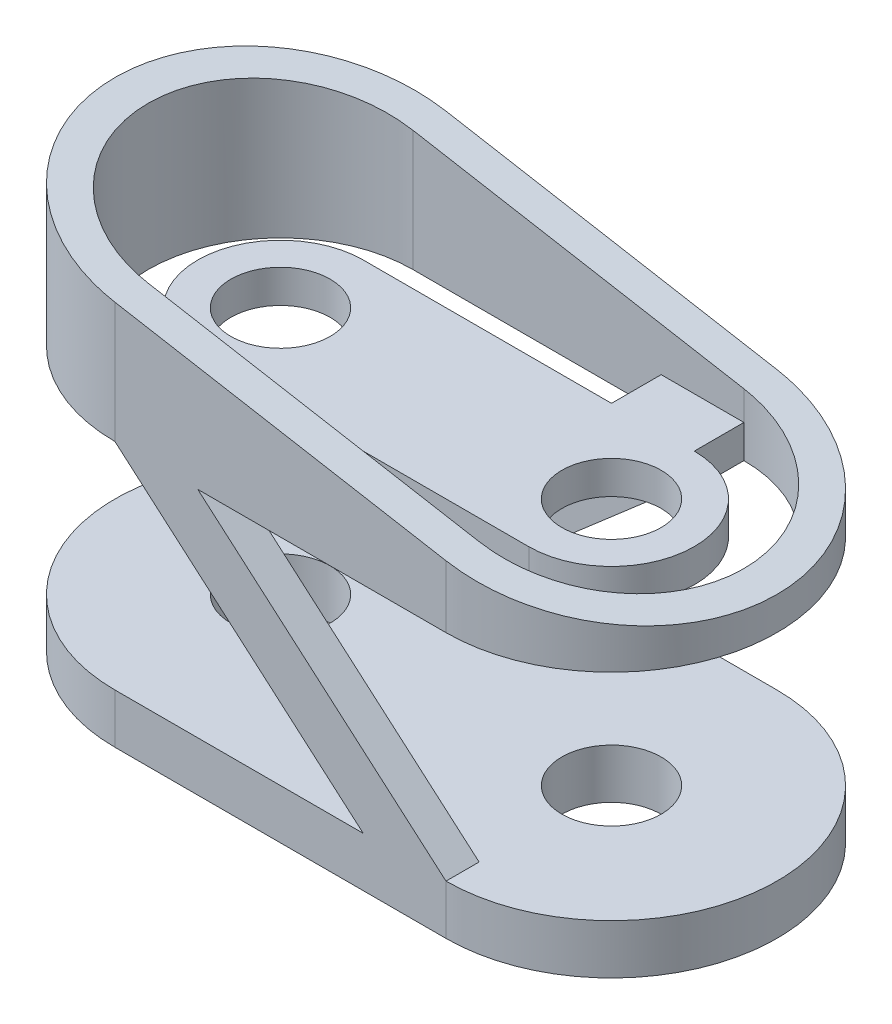
ISO-10303-21;
HEADER;
FILE_DESCRIPTION(('STEP AP214'),'2;1');
FILE_NAME('part.step','',(''),(''),'','','');
FILE_SCHEMA(('AUTOMOTIVE_DESIGN { 1 0 10303 214 1 1 1 1 }'));
ENDSEC;
DATA;
#1=APPLICATION_CONTEXT('core data for automotive mechanical design processes');
#2=APPLICATION_PROTOCOL_DEFINITION('international standard','automotive_design',2000,#1);
#3=PRODUCT_CONTEXT('',#1,'mechanical');
#4=PRODUCT('Part','Part','',(#3));
#5=PRODUCT_RELATED_PRODUCT_CATEGORY('part','',(#4));
#6=PRODUCT_DEFINITION_FORMATION('','',#4);
#7=PRODUCT_DEFINITION_CONTEXT('part definition',#1,'design');
#8=PRODUCT_DEFINITION('design','',#6,#7);
#9=PRODUCT_DEFINITION_SHAPE('','',#8);
#10=(LENGTH_UNIT() NAMED_UNIT(*) SI_UNIT(.MILLI.,.METRE.));
#11=(NAMED_UNIT(*) PLANE_ANGLE_UNIT() SI_UNIT($,.RADIAN.));
#12=(NAMED_UNIT(*) SI_UNIT($,.STERADIAN.) SOLID_ANGLE_UNIT());
#13=UNCERTAINTY_MEASURE_WITH_UNIT(LENGTH_MEASURE(1.E-05),#10,'distance_accuracy_value','');
#14=(GEOMETRIC_REPRESENTATION_CONTEXT(3) GLOBAL_UNCERTAINTY_ASSIGNED_CONTEXT((#13)) GLOBAL_UNIT_ASSIGNED_CONTEXT((#10,
#11,#12)) REPRESENTATION_CONTEXT('',''));
#15=CARTESIAN_POINT('',(0.,0.,0.));
#16=DIRECTION('',(0.,0.,1.));
#17=DIRECTION('',(1.,0.,0.));
#18=AXIS2_PLACEMENT_3D('',#15,#16,#17);
#19=CARTESIAN_POINT('',(-50.,90.,0.));
#20=DIRECTION('',(0.,1.,0.));
#21=DIRECTION('',(0.,0.,1.));
#22=AXIS2_PLACEMENT_3D('',#19,#20,#21);
#23=PLANE('',#22);
#24=CARTESIAN_POINT('',(50.,90.,0.));
#25=DIRECTION('',(0.,-1.,0.));
#26=DIRECTION('',(0.,0.,-1.));
#27=AXIS2_PLACEMENT_3D('',#24,#25,#26);
#28=CIRCLE('',#27,15.);
#29=CARTESIAN_POINT('',(50.,90.,-15.));
#30=VERTEX_POINT('',#29);
#31=EDGE_CURVE('E246',#30,#30,#28,.T.);
#32=ORIENTED_EDGE('',*,*,#31,.T.);
#33=EDGE_LOOP('',(#32));
#34=FACE_BOUND('',#33,.T.);
#35=CARTESIAN_POINT('',(-50.,90.,0.));
#36=DIRECTION('',(0.,-1.,0.));
#37=DIRECTION('',(0.,0.,-1.));
#38=AXIS2_PLACEMENT_3D('',#35,#36,#37);
#39=CIRCLE('',#38,15.);
#40=CARTESIAN_POINT('',(-50.,90.,-15.));
#41=VERTEX_POINT('',#40);
#42=EDGE_CURVE('E238',#41,#41,#39,.T.);
#43=ORIENTED_EDGE('',*,*,#42,.T.);
#44=EDGE_LOOP('',(#43));
#45=FACE_BOUND('',#44,.T.);
#46=DIRECTION('',(0.,0.,1.));
#47=VECTOR('',#46,1.);
#48=CARTESIAN_POINT('',(50.,90.,-25.));
#49=LINE('',#48,#47);
#50=CARTESIAN_POINT('',(50.,90.,-40.));
#51=VERTEX_POINT('',#50);
#52=CARTESIAN_POINT('',(50.,90.,-25.));
#53=VERTEX_POINT('',#52);
#54=EDGE_CURVE('E273',#51,#53,#49,.T.);
#55=ORIENTED_EDGE('',*,*,#54,.F.);
#56=DIRECTION('',(-1.,0.,0.));
#57=VECTOR('',#56,1.);
#58=CARTESIAN_POINT('',(50.,90.,-40.));
#59=LINE('',#58,#57);
#60=CARTESIAN_POINT('',(25.,90.,-40.));
#61=VERTEX_POINT('',#60);
#62=EDGE_CURVE('E237',#51,#61,#59,.T.);
#63=ORIENTED_EDGE('',*,*,#62,.T.);
#64=DIRECTION('',(0.,0.,-1.));
#65=VECTOR('',#64,1.);
#66=CARTESIAN_POINT('',(25.,90.,-25.));
#67=LINE('',#66,#65);
#68=CARTESIAN_POINT('',(25.,90.,-25.));
#69=VERTEX_POINT('',#68);
#70=EDGE_CURVE('E271',#69,#61,#67,.T.);
#71=ORIENTED_EDGE('',*,*,#70,.F.);
#72=DIRECTION('',(1.,0.,0.));
#73=VECTOR('',#72,1.);
#74=CARTESIAN_POINT('',(25.,90.,-25.));
#75=LINE('',#74,#73);
#76=CARTESIAN_POINT('',(-50.,90.,-25.));
#77=VERTEX_POINT('',#76);
#78=EDGE_CURVE('E268',#77,#69,#75,.T.);
#79=ORIENTED_EDGE('',*,*,#78,.F.);
#80=CARTESIAN_POINT('',(-50.,90.,0.));
#81=DIRECTION('',(0.,-1.,0.));
#82=DIRECTION('',(0.,0.,-1.));
#83=AXIS2_PLACEMENT_3D('',#80,#81,#82);
#84=CIRCLE('',#83,25.);
#85=CARTESIAN_POINT('',(-50.,90.,25.));
#86=VERTEX_POINT('',#85);
#87=EDGE_CURVE('E264',#86,#77,#84,.T.);
#88=ORIENTED_EDGE('',*,*,#87,.F.);
#89=DIRECTION('',(0.,0.,-1.));
#90=VECTOR('',#89,1.);
#91=CARTESIAN_POINT('',(-50.,90.,25.));
#92=LINE('',#91,#90);
#93=CARTESIAN_POINT('',(-50.,90.,40.));
#94=VERTEX_POINT('',#93);
#95=EDGE_CURVE('E265',#94,#86,#92,.T.);
#96=ORIENTED_EDGE('',*,*,#95,.F.);
#97=DIRECTION('',(1.,0.,0.));
#98=VECTOR('',#97,1.);
#99=CARTESIAN_POINT('',(50.,90.,40.));
#100=LINE('',#99,#98);
#101=CARTESIAN_POINT('',(-25.,90.,40.));
#102=VERTEX_POINT('',#101);
#103=EDGE_CURVE('E235',#94,#102,#100,.T.);
#104=ORIENTED_EDGE('',*,*,#103,.T.);
#105=DIRECTION('',(0.,0.,1.));
#106=VECTOR('',#105,1.);
#107=CARTESIAN_POINT('',(-25.,90.,40.));
#108=LINE('',#107,#106);
#109=CARTESIAN_POINT('',(-25.,90.,25.));
#110=VERTEX_POINT('',#109);
#111=EDGE_CURVE('E259',#110,#102,#108,.T.);
#112=ORIENTED_EDGE('',*,*,#111,.F.);
#113=DIRECTION('',(-1.,0.,0.));
#114=VECTOR('',#113,1.);
#115=CARTESIAN_POINT('',(50.,90.,25.));
#116=LINE('',#115,#114);
#117=CARTESIAN_POINT('',(50.,90.,25.));
#118=VERTEX_POINT('',#117);
#119=EDGE_CURVE('E254',#118,#110,#116,.T.);
#120=ORIENTED_EDGE('',*,*,#119,.F.);
#121=CARTESIAN_POINT('',(50.,90.,0.));
#122=DIRECTION('',(0.,-1.,0.));
#123=DIRECTION('',(0.,0.,-1.));
#124=AXIS2_PLACEMENT_3D('',#121,#122,#123);
#125=CIRCLE('',#124,25.);
#126=EDGE_CURVE('E252',#53,#118,#125,.T.);
#127=ORIENTED_EDGE('',*,*,#126,.F.);
#128=EDGE_LOOP('',(#55,#63,#71,#79,#88,#96,#104,#112,#120,#127));
#129=FACE_BOUND('',#128,.T.);
#130=ADVANCED_FACE('F39',(#34,#45,#129),#23,.T.);
#131=CARTESIAN_POINT('',(-50.,90.,40.));
#132=DIRECTION('',(0.,0.,-1.));
#133=DIRECTION('',(-1.,0.,0.));
#134=AXIS2_PLACEMENT_3D('',#131,#132,#133);
#135=PLANE('',#134);
#136=DIRECTION('',(0.,-1.,0.));
#137=VECTOR('',#136,1.);
#138=CARTESIAN_POINT('',(-25.,90.,40.));
#139=LINE('',#138,#137);
#140=CARTESIAN_POINT('',(-25.,80.,40.));
#141=VERTEX_POINT('',#140);
#142=EDGE_CURVE('E320',#102,#141,#139,.T.);
#143=ORIENTED_EDGE('',*,*,#142,.F.);
#144=ORIENTED_EDGE('',*,*,#103,.F.);
#145=DIRECTION('',(0.,-1.,0.));
#146=VECTOR('',#145,1.);
#147=CARTESIAN_POINT('',(-50.,332.964243462777,40.));
#148=LINE('',#147,#146);
#149=CARTESIAN_POINT('',(-50.,116.44904710627,40.));
#150=VERTEX_POINT('',#149);
#151=EDGE_CURVE('E221',#150,#94,#148,.T.);
#152=ORIENTED_EDGE('',*,*,#151,.F.);
#153=DIRECTION('',(0.984807753012208,-0.173648177666931,0.));
#154=VECTOR('',#153,1.);
#155=CARTESIAN_POINT('',(9.95835179427637,105.876771966129,40.));
#156=LINE('',#155,#154);
#157=CARTESIAN_POINT('',(50.,98.8163490354233,40.));
#158=VERTEX_POINT('',#157);
#159=EDGE_CURVE('E206',#150,#158,#156,.T.);
#160=ORIENTED_EDGE('',*,*,#159,.T.);
#161=DIRECTION('',(0.,-1.,0.));
#162=VECTOR('',#161,1.);
#163=CARTESIAN_POINT('',(50.,90.,40.));
#164=LINE('',#163,#162);
#165=CARTESIAN_POINT('',(50.,80.,40.));
#166=VERTEX_POINT('',#165);
#167=EDGE_CURVE('E356',#158,#166,#164,.T.);
#168=ORIENTED_EDGE('',*,*,#167,.T.);
#169=DIRECTION('',(1.,0.,0.));
#170=VECTOR('',#169,1.);
#171=CARTESIAN_POINT('',(-50.,80.,40.));
#172=LINE('',#171,#170);
#173=EDGE_CURVE('E344',#141,#166,#172,.T.);
#174=ORIENTED_EDGE('',*,*,#173,.F.);
#175=EDGE_LOOP('',(#143,#144,#152,#160,#168,#174));
#176=FACE_BOUND('',#175,.T.);
#177=ADVANCED_FACE('F231',(#176),#135,.T.);
#178=CARTESIAN_POINT('',(-50.,90.,-40.));
#179=DIRECTION('',(0.,0.,1.));
#180=DIRECTION('',(1.,0.,0.));
#181=AXIS2_PLACEMENT_3D('',#178,#179,#180);
#182=PLANE('',#181);
#183=DIRECTION('',(0.,-1.,0.));
#184=VECTOR('',#183,1.);
#185=CARTESIAN_POINT('',(25.,90.,-40.));
#186=LINE('',#185,#184);
#187=CARTESIAN_POINT('',(25.,80.,-40.));
#188=VERTEX_POINT('',#187);
#189=EDGE_CURVE('E306',#61,#188,#186,.T.);
#190=ORIENTED_EDGE('',*,*,#189,.F.);
#191=ORIENTED_EDGE('',*,*,#62,.F.);
#192=DIRECTION('',(0.,-1.,0.));
#193=VECTOR('',#192,1.);
#194=CARTESIAN_POINT('',(50.,332.964243462777,-40.));
#195=LINE('',#194,#193);
#196=CARTESIAN_POINT('',(50.,98.8163490354233,-40.));
#197=VERTEX_POINT('',#196);
#198=EDGE_CURVE('E217',#197,#51,#195,.T.);
#199=ORIENTED_EDGE('',*,*,#198,.F.);
#200=DIRECTION('',(-0.984807753012208,0.173648177666931,0.));
#201=VECTOR('',#200,1.);
#202=CARTESIAN_POINT('',(9.95835179427632,105.876771966129,-40.));
#203=LINE('',#202,#201);
#204=CARTESIAN_POINT('',(-50.,116.44904710627,-40.));
#205=VERTEX_POINT('',#204);
#206=EDGE_CURVE('E226',#197,#205,#203,.T.);
#207=ORIENTED_EDGE('',*,*,#206,.T.);
#208=DIRECTION('',(0.,-1.,0.));
#209=VECTOR('',#208,1.);
#210=CARTESIAN_POINT('',(-50.,90.,-40.));
#211=LINE('',#210,#209);
#212=CARTESIAN_POINT('',(-50.,80.,-40.));
#213=VERTEX_POINT('',#212);
#214=EDGE_CURVE('E230',#205,#213,#211,.T.);
#215=ORIENTED_EDGE('',*,*,#214,.T.);
#216=DIRECTION('',(-1.,0.,0.));
#217=VECTOR('',#216,1.);
#218=CARTESIAN_POINT('',(-50.,80.,-40.));
#219=LINE('',#218,#217);
#220=EDGE_CURVE('E348',#188,#213,#219,.T.);
#221=ORIENTED_EDGE('',*,*,#220,.F.);
#222=EDGE_LOOP('',(#190,#191,#199,#207,#215,#221));
#223=FACE_BOUND('',#222,.T.);
#224=ADVANCED_FACE('F502',(#223),#182,.T.);
#225=CARTESIAN_POINT('',(-50.,80.,0.));
#226=DIRECTION('',(0.,1.,0.));
#227=DIRECTION('',(0.,0.,1.));
#228=AXIS2_PLACEMENT_3D('',#225,#226,#227);
#229=PLANE('',#228);
#230=CARTESIAN_POINT('',(50.,80.,0.));
#231=DIRECTION('',(0.,1.,0.));
#232=DIRECTION('',(0.,0.,1.));
#233=AXIS2_PLACEMENT_3D('',#230,#231,#232);
#234=CIRCLE('',#233,40.);
#235=CARTESIAN_POINT('',(50.0000000000004,80.,-40.));
#236=VERTEX_POINT('',#235);
#237=EDGE_CURVE('E350',#166,#236,#234,.T.);
#238=ORIENTED_EDGE('',*,*,#237,.T.);
#239=DIRECTION('',(0.,0.,-1.));
#240=VECTOR('',#239,1.);
#241=CARTESIAN_POINT('',(50.,80.,79.2686044187656));
#242=LINE('',#241,#240);
#243=CARTESIAN_POINT('',(50.,80.,-50.));
#244=VERTEX_POINT('',#243);
#245=EDGE_CURVE('E336',#236,#244,#242,.T.);
#246=ORIENTED_EDGE('',*,*,#245,.T.);
#247=CARTESIAN_POINT('',(50.,80.,0.));
#248=DIRECTION('',(0.,1.,0.));
#249=DIRECTION('',(0.,0.,1.));
#250=AXIS2_PLACEMENT_3D('',#247,#248,#249);
#251=CIRCLE('',#250,50.);
#252=CARTESIAN_POINT('',(50.,80.,50.));
#253=VERTEX_POINT('',#252);
#254=EDGE_CURVE('E364',#253,#244,#251,.T.);
#255=ORIENTED_EDGE('',*,*,#254,.F.);
#256=DIRECTION('',(1.,0.,0.));
#257=VECTOR('',#256,1.);
#258=CARTESIAN_POINT('',(-50.,80.,50.));
#259=LINE('',#258,#257);
#260=CARTESIAN_POINT('',(-25.,80.,50.));
#261=VERTEX_POINT('',#260);
#262=EDGE_CURVE('E361',#261,#253,#259,.T.);
#263=ORIENTED_EDGE('',*,*,#262,.F.);
#264=DIRECTION('',(0.,0.,1.));
#265=VECTOR('',#264,1.);
#266=CARTESIAN_POINT('',(-25.,80.,-79.2686044187656));
#267=LINE('',#266,#265);
#268=EDGE_CURVE('E393',#141,#261,#267,.T.);
#269=ORIENTED_EDGE('',*,*,#268,.F.);
#270=ORIENTED_EDGE('',*,*,#173,.T.);
#271=EDGE_LOOP('',(#238,#246,#255,#263,#269,#270));
#272=FACE_BOUND('',#271,.T.);
#273=ADVANCED_FACE('F529',(#272),#229,.F.);
#274=CARTESIAN_POINT('',(-50.,15.,0.));
#275=DIRECTION('',(0.,1.,0.));
#276=DIRECTION('',(0.,0.,1.));
#277=AXIS2_PLACEMENT_3D('',#274,#275,#276);
#278=PLANE('',#277);
#279=DIRECTION('',(0.,0.,-1.));
#280=VECTOR('',#279,1.);
#281=CARTESIAN_POINT('',(-25.,15.,79.2686044187656));
#282=LINE('',#281,#280);
#283=CARTESIAN_POINT('',(-25.,15.,-40.));
#284=VERTEX_POINT('',#283);
#285=CARTESIAN_POINT('',(-25.,15.,-50.));
#286=VERTEX_POINT('',#285);
#287=EDGE_CURVE('E53',#284,#286,#282,.T.);
#288=ORIENTED_EDGE('',*,*,#287,.F.);
#289=DIRECTION('',(-1.,0.,0.));
#290=VECTOR('',#289,1.);
#291=CARTESIAN_POINT('',(-25.,15.,-40.));
#292=LINE('',#291,#290);
#293=CARTESIAN_POINT('',(-50.,15.,-40.));
#294=VERTEX_POINT('',#293);
#295=EDGE_CURVE('E59',#284,#294,#292,.T.);
#296=ORIENTED_EDGE('',*,*,#295,.T.);
#297=DIRECTION('',(0.,0.,-1.));
#298=VECTOR('',#297,1.);
#299=CARTESIAN_POINT('',(-50.,15.,79.2686044187656));
#300=LINE('',#299,#298);
#301=CARTESIAN_POINT('',(-50.,15.,-50.));
#302=VERTEX_POINT('',#301);
#303=EDGE_CURVE('E331',#294,#302,#300,.T.);
#304=ORIENTED_EDGE('',*,*,#303,.T.);
#305=CARTESIAN_POINT('',(-50.,15.,0.));
#306=DIRECTION('',(0.,1.,0.));
#307=DIRECTION('',(0.,0.,1.));
#308=AXIS2_PLACEMENT_3D('',#305,#306,#307);
#309=CIRCLE('',#308,50.);
#310=CARTESIAN_POINT('',(-50.,15.,50.));
#311=VERTEX_POINT('',#310);
#312=EDGE_CURVE('E419',#302,#311,#309,.T.);
#313=ORIENTED_EDGE('',*,*,#312,.T.);
#314=DIRECTION('',(1.,0.,0.));
#315=VECTOR('',#314,1.);
#316=CARTESIAN_POINT('',(-50.,15.,50.));
#317=LINE('',#316,#315);
#318=CARTESIAN_POINT('',(25.,15.,50.));
#319=VERTEX_POINT('',#318);
#320=EDGE_CURVE('E421',#311,#319,#317,.T.);
#321=ORIENTED_EDGE('',*,*,#320,.T.);
#322=DIRECTION('',(0.,0.,1.));
#323=VECTOR('',#322,1.);
#324=CARTESIAN_POINT('',(25.,15.,-79.2686044187656));
#325=LINE('',#324,#323);
#326=CARTESIAN_POINT('',(25.,15.,40.));
#327=VERTEX_POINT('',#326);
#328=EDGE_CURVE('E396',#327,#319,#325,.T.);
#329=ORIENTED_EDGE('',*,*,#328,.F.);
#330=DIRECTION('',(1.,0.,0.));
#331=VECTOR('',#330,1.);
#332=CARTESIAN_POINT('',(25.,15.,40.));
#333=LINE('',#332,#331);
#334=CARTESIAN_POINT('',(50.,15.,40.));
#335=VERTEX_POINT('',#334);
#336=EDGE_CURVE('E395',#327,#335,#333,.T.);
#337=ORIENTED_EDGE('',*,*,#336,.T.);
#338=DIRECTION('',(0.,0.,1.));
#339=VECTOR('',#338,1.);
#340=CARTESIAN_POINT('',(50.,15.,-79.2686044187656));
#341=LINE('',#340,#339);
#342=CARTESIAN_POINT('',(50.,15.,50.));
#343=VERTEX_POINT('',#342);
#344=EDGE_CURVE('E392',#335,#343,#341,.T.);
#345=ORIENTED_EDGE('',*,*,#344,.T.);
#346=CARTESIAN_POINT('',(50.,15.,0.));
#347=DIRECTION('',(0.,1.,0.));
#348=DIRECTION('',(0.,0.,1.));
#349=AXIS2_PLACEMENT_3D('',#346,#347,#348);
#350=CIRCLE('',#349,50.);
#351=CARTESIAN_POINT('',(50.,15.,-50.));
#352=VERTEX_POINT('',#351);
#353=EDGE_CURVE('E430',#343,#352,#350,.T.);
#354=ORIENTED_EDGE('',*,*,#353,.T.);
#355=DIRECTION('',(-1.,0.,0.));
#356=VECTOR('',#355,1.);
#357=CARTESIAN_POINT('',(-50.,15.,-50.));
#358=LINE('',#357,#356);
#359=EDGE_CURVE('E427',#352,#286,#358,.T.);
#360=ORIENTED_EDGE('',*,*,#359,.T.);
#361=EDGE_LOOP('',(#288,#296,#304,#313,#321,#329,#337,#345,#354,#360));
#362=FACE_BOUND('',#361,.T.);
#363=CARTESIAN_POINT('',(-50.,15.,0.));
#364=DIRECTION('',(0.,1.,0.));
#365=DIRECTION('',(0.,0.,1.));
#366=AXIS2_PLACEMENT_3D('',#363,#364,#365);
#367=CIRCLE('',#366,15.);
#368=CARTESIAN_POINT('',(-50.,15.,15.));
#369=VERTEX_POINT('',#368);
#370=EDGE_CURVE('E412',#369,#369,#367,.T.);
#371=ORIENTED_EDGE('',*,*,#370,.F.);
#372=EDGE_LOOP('',(#371));
#373=FACE_BOUND('',#372,.T.);
#374=CARTESIAN_POINT('',(50.,15.,0.));
#375=DIRECTION('',(0.,1.,0.));
#376=DIRECTION('',(0.,0.,1.));
#377=AXIS2_PLACEMENT_3D('',#374,#375,#376);
#378=CIRCLE('',#377,15.);
#379=CARTESIAN_POINT('',(50.,15.,15.));
#380=VERTEX_POINT('',#379);
#381=EDGE_CURVE('E406',#380,#380,#378,.T.);
#382=ORIENTED_EDGE('',*,*,#381,.F.);
#383=EDGE_LOOP('',(#382));
#384=FACE_BOUND('',#383,.T.);
#385=ADVANCED_FACE('F465',(#362,#373,#384),#278,.T.);
#386=CARTESIAN_POINT('',(-50.,0.,0.));
#387=DIRECTION('',(0.,1.,0.));
#388=DIRECTION('',(0.,0.,1.));
#389=AXIS2_PLACEMENT_3D('',#386,#387,#388);
#390=PLANE('',#389);
#391=CARTESIAN_POINT('',(-50.,0.,0.));
#392=DIRECTION('',(0.,1.,0.));
#393=DIRECTION('',(0.,0.,1.));
#394=AXIS2_PLACEMENT_3D('',#391,#392,#393);
#395=CIRCLE('',#394,50.);
#396=CARTESIAN_POINT('',(-50.,0.,-50.));
#397=VERTEX_POINT('',#396);
#398=CARTESIAN_POINT('',(-50.,0.,50.));
#399=VERTEX_POINT('',#398);
#400=EDGE_CURVE('E417',#397,#399,#395,.T.);
#401=ORIENTED_EDGE('',*,*,#400,.F.);
#402=DIRECTION('',(-1.,0.,0.));
#403=VECTOR('',#402,1.);
#404=CARTESIAN_POINT('',(-50.,0.,-50.));
#405=LINE('',#404,#403);
#406=CARTESIAN_POINT('',(50.,0.,-50.));
#407=VERTEX_POINT('',#406);
#408=EDGE_CURVE('E424',#407,#397,#405,.T.);
#409=ORIENTED_EDGE('',*,*,#408,.F.);
#410=CARTESIAN_POINT('',(50.,0.,0.));
#411=DIRECTION('',(0.,1.,0.));
#412=DIRECTION('',(0.,0.,1.));
#413=AXIS2_PLACEMENT_3D('',#410,#411,#412);
#414=CIRCLE('',#413,50.);
#415=CARTESIAN_POINT('',(50.,0.,50.));
#416=VERTEX_POINT('',#415);
#417=EDGE_CURVE('E436',#416,#407,#414,.T.);
#418=ORIENTED_EDGE('',*,*,#417,.F.);
#419=DIRECTION('',(1.,0.,0.));
#420=VECTOR('',#419,1.);
#421=CARTESIAN_POINT('',(-50.,0.,50.));
#422=LINE('',#421,#420);
#423=EDGE_CURVE('E432',#399,#416,#422,.T.);
#424=ORIENTED_EDGE('',*,*,#423,.F.);
#425=EDGE_LOOP('',(#401,#409,#418,#424));
#426=FACE_BOUND('',#425,.T.);
#427=CARTESIAN_POINT('',(-50.,0.,0.));
#428=DIRECTION('',(0.,1.,0.));
#429=DIRECTION('',(0.,0.,1.));
#430=AXIS2_PLACEMENT_3D('',#427,#428,#429);
#431=CIRCLE('',#430,15.);
#432=CARTESIAN_POINT('',(-50.,0.,15.));
#433=VERTEX_POINT('',#432);
#434=EDGE_CURVE('E411',#433,#433,#431,.T.);
#435=ORIENTED_EDGE('',*,*,#434,.T.);
#436=EDGE_LOOP('',(#435));
#437=FACE_BOUND('',#436,.T.);
#438=CARTESIAN_POINT('',(50.,0.,0.));
#439=DIRECTION('',(0.,1.,0.));
#440=DIRECTION('',(0.,0.,1.));
#441=AXIS2_PLACEMENT_3D('',#438,#439,#440);
#442=CIRCLE('',#441,15.);
#443=CARTESIAN_POINT('',(50.,0.,15.));
#444=VERTEX_POINT('',#443);
#445=EDGE_CURVE('E410',#444,#444,#442,.T.);
#446=ORIENTED_EDGE('',*,*,#445,.T.);
#447=EDGE_LOOP('',(#446));
#448=FACE_BOUND('',#447,.T.);
#449=ADVANCED_FACE('F452',(#426,#437,#448),#390,.F.);
#450=CARTESIAN_POINT('',(-50.,15.,0.));
#451=DIRECTION('',(0.,-1.,0.));
#452=DIRECTION('',(0.,0.,-1.));
#453=AXIS2_PLACEMENT_3D('',#450,#451,#452);
#454=CYLINDRICAL_SURFACE('',#453,50.);
#455=ORIENTED_EDGE('',*,*,#400,.T.);
#456=DIRECTION('',(0.,-1.,0.));
#457=VECTOR('',#456,1.);
#458=CARTESIAN_POINT('',(-50.,15.,50.));
#459=LINE('',#458,#457);
#460=EDGE_CURVE('E11',#311,#399,#459,.T.);
#461=ORIENTED_EDGE('',*,*,#460,.F.);
#462=ORIENTED_EDGE('',*,*,#312,.F.);
#463=DIRECTION('',(0.,-1.,0.));
#464=VECTOR('',#463,1.);
#465=CARTESIAN_POINT('',(-50.,15.,-50.));
#466=LINE('',#465,#464);
#467=EDGE_CURVE('E431',#302,#397,#466,.T.);
#468=ORIENTED_EDGE('',*,*,#467,.T.);
#469=EDGE_LOOP('',(#455,#461,#462,#468));
#470=FACE_BOUND('',#469,.T.);
#471=ADVANCED_FACE('F41',(#470),#454,.T.);
#472=CARTESIAN_POINT('',(-50.,15.,50.));
#473=DIRECTION('',(0.,0.,-1.));
#474=DIRECTION('',(-1.,0.,0.));
#475=AXIS2_PLACEMENT_3D('',#472,#473,#474);
#476=PLANE('',#475);
#477=ORIENTED_EDGE('',*,*,#423,.T.);
#478=DIRECTION('',(0.,-1.,0.));
#479=VECTOR('',#478,1.);
#480=CARTESIAN_POINT('',(50.,15.,50.));
#481=LINE('',#480,#479);
#482=EDGE_CURVE('E50',#343,#416,#481,.T.);
#483=ORIENTED_EDGE('',*,*,#482,.F.);
#484=DIRECTION('',(-0.755689082789818,0.654930538417842,0.));
#485=VECTOR('',#484,1.);
#486=CARTESIAN_POINT('',(50.,15.,50.));
#487=LINE('',#486,#485);
#488=EDGE_CURVE('E385',#343,#261,#487,.T.);
#489=ORIENTED_EDGE('',*,*,#488,.T.);
#490=ORIENTED_EDGE('',*,*,#262,.T.);
#491=DIRECTION('',(0.,-1.,0.));
#492=VECTOR('',#491,1.);
#493=CARTESIAN_POINT('',(50.,90.,50.));
#494=LINE('',#493,#492);
#495=CARTESIAN_POINT('',(50.,98.8163490354233,50.));
#496=VERTEX_POINT('',#495);
#497=EDGE_CURVE('E376',#496,#253,#494,.T.);
#498=ORIENTED_EDGE('',*,*,#497,.F.);
#499=DIRECTION('',(0.984807753012208,-0.173648177666931,0.));
#500=VECTOR('',#499,1.);
#501=CARTESIAN_POINT('',(-87.0262792450191,122.977779132413,50.));
#502=LINE('',#501,#500);
#503=CARTESIAN_POINT('',(-50.,116.44904710627,50.));
#504=VERTEX_POINT('',#503);
#505=EDGE_CURVE('E484',#504,#496,#502,.T.);
#506=ORIENTED_EDGE('',*,*,#505,.F.);
#507=DIRECTION('',(0.,-1.,0.));
#508=VECTOR('',#507,1.);
#509=CARTESIAN_POINT('',(-50.,90.,50.));
#510=LINE('',#509,#508);
#511=CARTESIAN_POINT('',(-50.,80.,50.));
#512=VERTEX_POINT('',#511);
#513=EDGE_CURVE('E377',#504,#512,#510,.T.);
#514=ORIENTED_EDGE('',*,*,#513,.T.);
#515=DIRECTION('',(0.755689082789818,-0.654930538417842,0.));
#516=VECTOR('',#515,1.);
#517=CARTESIAN_POINT('',(25.,15.,50.));
#518=LINE('',#517,#516);
#519=EDGE_CURVE('E382',#512,#319,#518,.T.);
#520=ORIENTED_EDGE('',*,*,#519,.T.);
#521=ORIENTED_EDGE('',*,*,#320,.F.);
#522=ORIENTED_EDGE('',*,*,#460,.T.);
#523=EDGE_LOOP('',(#477,#483,#489,#490,#498,#506,#514,#520,#521,#522));
#524=FACE_BOUND('',#523,.T.);
#525=ADVANCED_FACE('F483',(#524),#476,.F.);
#526=CARTESIAN_POINT('',(50.,15.,0.));
#527=DIRECTION('',(0.,-1.,0.));
#528=DIRECTION('',(0.,0.,-1.));
#529=AXIS2_PLACEMENT_3D('',#526,#527,#528);
#530=CYLINDRICAL_SURFACE('',#529,50.);
#531=ORIENTED_EDGE('',*,*,#417,.T.);
#532=DIRECTION('',(0.,-1.,0.));
#533=VECTOR('',#532,1.);
#534=CARTESIAN_POINT('',(50.,15.,-50.));
#535=LINE('',#534,#533);
#536=EDGE_CURVE('E442',#352,#407,#535,.T.);
#537=ORIENTED_EDGE('',*,*,#536,.F.);
#538=ORIENTED_EDGE('',*,*,#353,.F.);
#539=ORIENTED_EDGE('',*,*,#482,.T.);
#540=EDGE_LOOP('',(#531,#537,#538,#539));
#541=FACE_BOUND('',#540,.T.);
#542=ADVANCED_FACE('F446',(#541),#530,.T.);
#543=CARTESIAN_POINT('',(-50.,15.,-50.));
#544=DIRECTION('',(0.,0.,1.));
#545=DIRECTION('',(1.,0.,0.));
#546=AXIS2_PLACEMENT_3D('',#543,#544,#545);
#547=PLANE('',#546);
#548=ORIENTED_EDGE('',*,*,#408,.T.);
#549=ORIENTED_EDGE('',*,*,#467,.F.);
#550=DIRECTION('',(0.755689082789818,0.654930538417842,0.));
#551=VECTOR('',#550,1.);
#552=CARTESIAN_POINT('',(-50.,15.,-50.));
#553=LINE('',#552,#551);
#554=CARTESIAN_POINT('',(25.,80.,-50.));
#555=VERTEX_POINT('',#554);
#556=EDGE_CURVE('E325',#302,#555,#553,.T.);
#557=ORIENTED_EDGE('',*,*,#556,.T.);
#558=DIRECTION('',(-1.,0.,0.));
#559=VECTOR('',#558,1.);
#560=CARTESIAN_POINT('',(-50.,80.,-50.));
#561=LINE('',#560,#559);
#562=CARTESIAN_POINT('',(-50.,80.,-50.));
#563=VERTEX_POINT('',#562);
#564=EDGE_CURVE('E366',#555,#563,#561,.T.);
#565=ORIENTED_EDGE('',*,*,#564,.T.);
#566=DIRECTION('',(0.,-1.,0.));
#567=VECTOR('',#566,1.);
#568=CARTESIAN_POINT('',(-50.,90.,-50.));
#569=LINE('',#568,#567);
#570=CARTESIAN_POINT('',(-50.,116.44904710627,-50.));
#571=VERTEX_POINT('',#570);
#572=EDGE_CURVE('E367',#571,#563,#569,.T.);
#573=ORIENTED_EDGE('',*,*,#572,.F.);
#574=DIRECTION('',(-0.984807753012208,0.173648177666931,0.));
#575=VECTOR('',#574,1.);
#576=CARTESIAN_POINT('',(9.95835179427634,105.876771966129,-50.));
#577=LINE('',#576,#575);
#578=CARTESIAN_POINT('',(50.,98.8163490354233,-50.));
#579=VERTEX_POINT('',#578);
#580=EDGE_CURVE('E488',#579,#571,#577,.T.);
#581=ORIENTED_EDGE('',*,*,#580,.F.);
#582=DIRECTION('',(0.,-1.,0.));
#583=VECTOR('',#582,1.);
#584=CARTESIAN_POINT('',(50.,90.,-50.));
#585=LINE('',#584,#583);
#586=EDGE_CURVE('E373',#579,#244,#585,.T.);
#587=ORIENTED_EDGE('',*,*,#586,.T.);
#588=DIRECTION('',(-0.755689082789818,-0.654930538417842,0.));
#589=VECTOR('',#588,1.);
#590=CARTESIAN_POINT('',(50.,80.,-50.));
#591=LINE('',#590,#589);
#592=EDGE_CURVE('E307',#244,#286,#591,.T.);
#593=ORIENTED_EDGE('',*,*,#592,.T.);
#594=ORIENTED_EDGE('',*,*,#359,.F.);
#595=ORIENTED_EDGE('',*,*,#536,.T.);
#596=EDGE_LOOP('',(#548,#549,#557,#565,#573,#581,#587,#593,#594,#595));
#597=FACE_BOUND('',#596,.T.);
#598=ADVANCED_FACE('F456',(#597),#547,.F.);
#599=CARTESIAN_POINT('',(-50.,15.,0.));
#600=DIRECTION('',(0.,-1.,0.));
#601=DIRECTION('',(0.,0.,-1.));
#602=AXIS2_PLACEMENT_3D('',#599,#600,#601);
#603=CYLINDRICAL_SURFACE('',#602,15.);
#604=ORIENTED_EDGE('',*,*,#370,.T.);
#605=EDGE_LOOP('',(#604));
#606=FACE_BOUND('',#605,.T.);
#607=ORIENTED_EDGE('',*,*,#434,.F.);
#608=EDGE_LOOP('',(#607));
#609=FACE_BOUND('',#608,.T.);
#610=ADVANCED_FACE('F598',(#606,#609),#603,.F.);
#611=CARTESIAN_POINT('',(50.,15.,0.));
#612=DIRECTION('',(0.,-1.,0.));
#613=DIRECTION('',(0.,0.,-1.));
#614=AXIS2_PLACEMENT_3D('',#611,#612,#613);
#615=CYLINDRICAL_SURFACE('',#614,15.);
#616=ORIENTED_EDGE('',*,*,#381,.T.);
#617=EDGE_LOOP('',(#616));
#618=FACE_BOUND('',#617,.T.);
#619=ORIENTED_EDGE('',*,*,#445,.F.);
#620=EDGE_LOOP('',(#619));
#621=FACE_BOUND('',#620,.T.);
#622=ADVANCED_FACE('F592',(#618,#621),#615,.F.);
#623=DIRECTION('',(-1.,0.,0.));
#624=VECTOR('',#623,1.);
#625=CARTESIAN_POINT('',(-50.0000000000001,80.,40.));
#626=LINE('',#625,#624);
#627=CARTESIAN_POINT('',(-50.,80.,40.));
#628=VERTEX_POINT('',#627);
#629=EDGE_CURVE('E286',#141,#628,#626,.T.);
#630=ORIENTED_EDGE('',*,*,#629,.F.);
#631=DIRECTION('',(-0.755689082789818,0.654930538417842,0.));
#632=VECTOR('',#631,1.);
#633=CARTESIAN_POINT('',(50.,15.,40.));
#634=LINE('',#633,#632);
#635=EDGE_CURVE('E387',#335,#141,#634,.T.);
#636=ORIENTED_EDGE('',*,*,#635,.F.);
#637=ORIENTED_EDGE('',*,*,#336,.F.);
#638=DIRECTION('',(0.755689082789818,-0.654930538417842,0.));
#639=VECTOR('',#638,1.);
#640=CARTESIAN_POINT('',(25.,15.,40.));
#641=LINE('',#640,#639);
#642=EDGE_CURVE('E400',#628,#327,#641,.T.);
#643=ORIENTED_EDGE('',*,*,#642,.F.);
#644=EDGE_LOOP('',(#630,#636,#637,#643));
#645=FACE_BOUND('',#644,.T.);
#646=ADVANCED_FACE('F580',(#645),#135,.T.);
#647=CARTESIAN_POINT('',(50.,15.,-79.2686044187656));
#648=DIRECTION('',(0.654930538417842,0.755689082789818,0.));
#649=DIRECTION('',(-0.755689082789818,0.654930538417842,0.));
#650=AXIS2_PLACEMENT_3D('',#647,#648,#649);
#651=PLANE('',#650);
#652=ORIENTED_EDGE('',*,*,#344,.F.);
#653=ORIENTED_EDGE('',*,*,#635,.T.);
#654=ORIENTED_EDGE('',*,*,#268,.T.);
#655=ORIENTED_EDGE('',*,*,#488,.F.);
#656=EDGE_LOOP('',(#652,#653,#654,#655));
#657=FACE_BOUND('',#656,.T.);
#658=ADVANCED_FACE('F532',(#657),#651,.T.);
#659=CARTESIAN_POINT('',(25.,15.,-79.2686044187656));
#660=DIRECTION('',(-0.654930538417842,-0.755689082789818,0.));
#661=DIRECTION('',(0.755689082789818,-0.654930538417842,0.));
#662=AXIS2_PLACEMENT_3D('',#659,#660,#661);
#663=PLANE('',#662);
#664=DIRECTION('',(0.,0.,1.));
#665=VECTOR('',#664,1.);
#666=CARTESIAN_POINT('',(-50.,80.,-79.2686044187656));
#667=LINE('',#666,#665);
#668=EDGE_CURVE('E399',#628,#512,#667,.T.);
#669=ORIENTED_EDGE('',*,*,#668,.F.);
#670=ORIENTED_EDGE('',*,*,#642,.T.);
#671=ORIENTED_EDGE('',*,*,#328,.T.);
#672=ORIENTED_EDGE('',*,*,#519,.F.);
#673=EDGE_LOOP('',(#669,#670,#671,#672));
#674=FACE_BOUND('',#673,.T.);
#675=ADVANCED_FACE('F585',(#674),#663,.T.);
#676=ORIENTED_EDGE('',*,*,#564,.F.);
#677=DIRECTION('',(0.,0.,-1.));
#678=VECTOR('',#677,1.);
#679=CARTESIAN_POINT('',(25.,80.,79.2686044187656));
#680=LINE('',#679,#678);
#681=EDGE_CURVE('E334',#188,#555,#680,.T.);
#682=ORIENTED_EDGE('',*,*,#681,.F.);
#683=ORIENTED_EDGE('',*,*,#220,.T.);
#684=CARTESIAN_POINT('',(-50.,80.,0.));
#685=DIRECTION('',(0.,1.,0.));
#686=DIRECTION('',(0.,0.,1.));
#687=AXIS2_PLACEMENT_3D('',#684,#685,#686);
#688=CIRCLE('',#687,40.);
#689=EDGE_CURVE('E345',#213,#628,#688,.T.);
#690=ORIENTED_EDGE('',*,*,#689,.T.);
#691=ORIENTED_EDGE('',*,*,#668,.T.);
#692=CARTESIAN_POINT('',(-50.,80.,0.));
#693=DIRECTION('',(0.,1.,0.));
#694=DIRECTION('',(0.,0.,1.));
#695=AXIS2_PLACEMENT_3D('',#692,#693,#694);
#696=CIRCLE('',#695,50.);
#697=EDGE_CURVE('E359',#563,#512,#696,.T.);
#698=ORIENTED_EDGE('',*,*,#697,.F.);
#699=EDGE_LOOP('',(#676,#682,#683,#690,#691,#698));
#700=FACE_BOUND('',#699,.T.);
#701=ADVANCED_FACE('F479',(#700),#229,.F.);
#702=CARTESIAN_POINT('',(-50.,90.,0.));
#703=DIRECTION('',(0.,-1.,0.));
#704=DIRECTION('',(0.,0.,-1.));
#705=AXIS2_PLACEMENT_3D('',#702,#703,#704);
#706=CYLINDRICAL_SURFACE('',#705,50.);
#707=ORIENTED_EDGE('',*,*,#697,.T.);
#708=ORIENTED_EDGE('',*,*,#513,.F.);
#709=CARTESIAN_POINT('',(-50.,116.44904710627,0.));
#710=DIRECTION('',(0.173648177666931,0.984807753012208,0.));
#711=DIRECTION('',(0.984807753012208,-0.173648177666931,0.));
#712=AXIS2_PLACEMENT_3D('',#709,#710,#711);
#713=ELLIPSE('',#712,50.7713305942873,50.);
#714=EDGE_CURVE('E480',#571,#504,#713,.T.);
#715=ORIENTED_EDGE('',*,*,#714,.F.);
#716=ORIENTED_EDGE('',*,*,#572,.T.);
#717=EDGE_LOOP('',(#707,#708,#715,#716));
#718=FACE_BOUND('',#717,.T.);
#719=ADVANCED_FACE('F474',(#718),#706,.T.);
#720=CARTESIAN_POINT('',(50.,90.,0.));
#721=DIRECTION('',(0.,-1.,0.));
#722=DIRECTION('',(0.,0.,-1.));
#723=AXIS2_PLACEMENT_3D('',#720,#721,#722);
#724=CYLINDRICAL_SURFACE('',#723,50.);
#725=ORIENTED_EDGE('',*,*,#254,.T.);
#726=ORIENTED_EDGE('',*,*,#586,.F.);
#727=CARTESIAN_POINT('',(50.,98.8163490354233,0.));
#728=DIRECTION('',(0.173648177666931,0.984807753012208,0.));
#729=DIRECTION('',(0.984807753012208,-0.173648177666931,0.));
#730=AXIS2_PLACEMENT_3D('',#727,#728,#729);
#731=ELLIPSE('',#730,50.7713305942873,50.);
#732=EDGE_CURVE('E489',#496,#579,#731,.T.);
#733=ORIENTED_EDGE('',*,*,#732,.F.);
#734=ORIENTED_EDGE('',*,*,#497,.T.);
#735=EDGE_LOOP('',(#725,#726,#733,#734));
#736=FACE_BOUND('',#735,.T.);
#737=ADVANCED_FACE('F540',(#736),#724,.T.);
#738=CARTESIAN_POINT('',(-50.,90.,0.));
#739=DIRECTION('',(0.,-1.,0.));
#740=DIRECTION('',(0.,0.,-1.));
#741=AXIS2_PLACEMENT_3D('',#738,#739,#740);
#742=CYLINDRICAL_SURFACE('',#741,40.);
#743=ORIENTED_EDGE('',*,*,#689,.F.);
#744=ORIENTED_EDGE('',*,*,#214,.F.);
#745=CARTESIAN_POINT('',(-50.,116.44904710627,0.));
#746=DIRECTION('',(0.173648177666931,0.984807753012208,0.));
#747=DIRECTION('',(0.984807753012208,-0.173648177666931,0.));
#748=AXIS2_PLACEMENT_3D('',#745,#746,#747);
#749=ELLIPSE('',#748,40.6170644754298,40.);
#750=EDGE_CURVE('E209',#205,#150,#749,.T.);
#751=ORIENTED_EDGE('',*,*,#750,.T.);
#752=ORIENTED_EDGE('',*,*,#151,.T.);
#753=DIRECTION('',(0.,-1.,0.));
#754=VECTOR('',#753,1.);
#755=CARTESIAN_POINT('',(-50.,90.,40.));
#756=LINE('',#755,#754);
#757=EDGE_CURVE('E358',#94,#628,#756,.T.);
#758=ORIENTED_EDGE('',*,*,#757,.T.);
#759=EDGE_LOOP('',(#743,#744,#751,#752,#758));
#760=FACE_BOUND('',#759,.T.);
#761=ADVANCED_FACE('F225',(#760),#742,.F.);
#762=CARTESIAN_POINT('',(50.,90.,0.));
#763=DIRECTION('',(0.,-1.,0.));
#764=DIRECTION('',(0.,0.,-1.));
#765=AXIS2_PLACEMENT_3D('',#762,#763,#764);
#766=CYLINDRICAL_SURFACE('',#765,40.);
#767=ORIENTED_EDGE('',*,*,#237,.F.);
#768=ORIENTED_EDGE('',*,*,#167,.F.);
#769=CARTESIAN_POINT('',(50.,98.8163490354233,0.));
#770=DIRECTION('',(0.173648177666931,0.984807753012208,0.));
#771=DIRECTION('',(0.984807753012208,-0.173648177666931,0.));
#772=AXIS2_PLACEMENT_3D('',#769,#770,#771);
#773=ELLIPSE('',#772,40.6170644754298,40.);
#774=EDGE_CURVE('E213',#158,#197,#773,.T.);
#775=ORIENTED_EDGE('',*,*,#774,.T.);
#776=ORIENTED_EDGE('',*,*,#198,.T.);
#777=DIRECTION('',(0.,-1.,0.));
#778=VECTOR('',#777,1.);
#779=CARTESIAN_POINT('',(50.,90.,-40.));
#780=LINE('',#779,#778);
#781=EDGE_CURVE('E351',#51,#236,#780,.T.);
#782=ORIENTED_EDGE('',*,*,#781,.T.);
#783=EDGE_LOOP('',(#767,#768,#775,#776,#782));
#784=FACE_BOUND('',#783,.T.);
#785=ADVANCED_FACE('F681',(#784),#766,.F.);
#786=DIRECTION('',(1.,0.,0.));
#787=VECTOR('',#786,1.);
#788=CARTESIAN_POINT('',(50.0000000000004,80.,-40.));
#789=LINE('',#788,#787);
#790=EDGE_CURVE('E297',#188,#236,#789,.T.);
#791=ORIENTED_EDGE('',*,*,#790,.F.);
#792=DIRECTION('',(0.755689082789818,0.654930538417842,0.));
#793=VECTOR('',#792,1.);
#794=CARTESIAN_POINT('',(-50.,15.,-40.));
#795=LINE('',#794,#793);
#796=EDGE_CURVE('E329',#294,#188,#795,.T.);
#797=ORIENTED_EDGE('',*,*,#796,.F.);
#798=ORIENTED_EDGE('',*,*,#295,.F.);
#799=DIRECTION('',(-0.755689082789818,-0.654930538417842,0.));
#800=VECTOR('',#799,1.);
#801=CARTESIAN_POINT('',(50.,80.,-40.));
#802=LINE('',#801,#800);
#803=EDGE_CURVE('E324',#236,#284,#802,.T.);
#804=ORIENTED_EDGE('',*,*,#803,.F.);
#805=EDGE_LOOP('',(#791,#797,#798,#804));
#806=FACE_BOUND('',#805,.T.);
#807=ADVANCED_FACE('F542',(#806),#182,.T.);
#808=CARTESIAN_POINT('',(50.,80.,79.2686044187656));
#809=DIRECTION('',(0.654930538417842,-0.755689082789818,0.));
#810=DIRECTION('',(0.755689082789818,0.654930538417842,0.));
#811=AXIS2_PLACEMENT_3D('',#808,#809,#810);
#812=PLANE('',#811);
#813=ORIENTED_EDGE('',*,*,#245,.F.);
#814=ORIENTED_EDGE('',*,*,#803,.T.);
#815=ORIENTED_EDGE('',*,*,#287,.T.);
#816=ORIENTED_EDGE('',*,*,#592,.F.);
#817=EDGE_LOOP('',(#813,#814,#815,#816));
#818=FACE_BOUND('',#817,.T.);
#819=ADVANCED_FACE('F545',(#818),#812,.T.);
#820=CARTESIAN_POINT('',(-50.,15.,79.2686044187656));
#821=DIRECTION('',(-0.654930538417842,0.755689082789818,0.));
#822=DIRECTION('',(-0.755689082789818,-0.654930538417842,0.));
#823=AXIS2_PLACEMENT_3D('',#820,#821,#822);
#824=PLANE('',#823);
#825=ORIENTED_EDGE('',*,*,#303,.F.);
#826=ORIENTED_EDGE('',*,*,#796,.T.);
#827=ORIENTED_EDGE('',*,*,#681,.T.);
#828=ORIENTED_EDGE('',*,*,#556,.F.);
#829=EDGE_LOOP('',(#825,#826,#827,#828));
#830=FACE_BOUND('',#829,.T.);
#831=ADVANCED_FACE('F468',(#830),#824,.T.);
#832=CARTESIAN_POINT('',(50.,90.,0.));
#833=DIRECTION('',(0.,-1.,0.));
#834=DIRECTION('',(0.,0.,-1.));
#835=AXIS2_PLACEMENT_3D('',#832,#833,#834);
#836=CYLINDRICAL_SURFACE('',#835,25.);
#837=CARTESIAN_POINT('',(50.,80.,0.));
#838=DIRECTION('',(0.,-1.,0.));
#839=DIRECTION('',(0.,0.,-1.));
#840=AXIS2_PLACEMENT_3D('',#837,#838,#839);
#841=CIRCLE('',#840,25.);
#842=CARTESIAN_POINT('',(50.,80.,-25.));
#843=VERTEX_POINT('',#842);
#844=CARTESIAN_POINT('',(50.,80.,25.));
#845=VERTEX_POINT('',#844);
#846=EDGE_CURVE('E247',#843,#845,#841,.T.);
#847=ORIENTED_EDGE('',*,*,#846,.F.);
#848=DIRECTION('',(0.,-1.,0.));
#849=VECTOR('',#848,1.);
#850=CARTESIAN_POINT('',(50.,90.,-25.));
#851=LINE('',#850,#849);
#852=EDGE_CURVE('E304',#53,#843,#851,.T.);
#853=ORIENTED_EDGE('',*,*,#852,.F.);
#854=ORIENTED_EDGE('',*,*,#126,.T.);
#855=DIRECTION('',(0.,-1.,0.));
#856=VECTOR('',#855,1.);
#857=CARTESIAN_POINT('',(50.,90.,25.));
#858=LINE('',#857,#856);
#859=EDGE_CURVE('E280',#118,#845,#858,.T.);
#860=ORIENTED_EDGE('',*,*,#859,.T.);
#861=EDGE_LOOP('',(#847,#853,#854,#860));
#862=FACE_BOUND('',#861,.T.);
#863=ADVANCED_FACE('F555',(#862),#836,.T.);
#864=CARTESIAN_POINT('',(50.,90.,-25.));
#865=DIRECTION('',(1.,0.,0.));
#866=DIRECTION('',(0.,0.,-1.));
#867=AXIS2_PLACEMENT_3D('',#864,#865,#866);
#868=PLANE('',#867);
#869=DIRECTION('',(0.,0.,1.));
#870=VECTOR('',#869,1.);
#871=CARTESIAN_POINT('',(50.,80.,-25.));
#872=LINE('',#871,#870);
#873=EDGE_CURVE('E258',#236,#843,#872,.T.);
#874=ORIENTED_EDGE('',*,*,#873,.F.);
#875=ORIENTED_EDGE('',*,*,#781,.F.);
#876=ORIENTED_EDGE('',*,*,#54,.T.);
#877=ORIENTED_EDGE('',*,*,#852,.T.);
#878=EDGE_LOOP('',(#874,#875,#876,#877));
#879=FACE_BOUND('',#878,.T.);
#880=ADVANCED_FACE('F548',(#879),#868,.T.);
#881=CARTESIAN_POINT('',(25.,90.,-25.));
#882=DIRECTION('',(-1.,0.,0.));
#883=DIRECTION('',(0.,0.,1.));
#884=AXIS2_PLACEMENT_3D('',#881,#882,#883);
#885=PLANE('',#884);
#886=DIRECTION('',(0.,0.,-1.));
#887=VECTOR('',#886,1.);
#888=CARTESIAN_POINT('',(25.,80.,-25.));
#889=LINE('',#888,#887);
#890=CARTESIAN_POINT('',(25.,80.,-25.));
#891=VERTEX_POINT('',#890);
#892=EDGE_CURVE('E300',#891,#188,#889,.T.);
#893=ORIENTED_EDGE('',*,*,#892,.F.);
#894=DIRECTION('',(0.,-1.,0.));
#895=VECTOR('',#894,1.);
#896=CARTESIAN_POINT('',(25.,90.,-25.));
#897=LINE('',#896,#895);
#898=EDGE_CURVE('E313',#69,#891,#897,.T.);
#899=ORIENTED_EDGE('',*,*,#898,.F.);
#900=ORIENTED_EDGE('',*,*,#70,.T.);
#901=ORIENTED_EDGE('',*,*,#189,.T.);
#902=EDGE_LOOP('',(#893,#899,#900,#901));
#903=FACE_BOUND('',#902,.T.);
#904=ADVANCED_FACE('F508',(#903),#885,.T.);
#905=CARTESIAN_POINT('',(25.,90.,-25.));
#906=DIRECTION('',(0.,0.,-1.));
#907=DIRECTION('',(-1.,0.,0.));
#908=AXIS2_PLACEMENT_3D('',#905,#906,#907);
#909=PLANE('',#908);
#910=DIRECTION('',(1.,0.,0.));
#911=VECTOR('',#910,1.);
#912=CARTESIAN_POINT('',(25.,80.,-25.));
#913=LINE('',#912,#911);
#914=CARTESIAN_POINT('',(-50.,80.,-25.));
#915=VERTEX_POINT('',#914);
#916=EDGE_CURVE('E294',#915,#891,#913,.T.);
#917=ORIENTED_EDGE('',*,*,#916,.F.);
#918=DIRECTION('',(0.,-1.,0.));
#919=VECTOR('',#918,1.);
#920=CARTESIAN_POINT('',(-50.,90.,-25.));
#921=LINE('',#920,#919);
#922=EDGE_CURVE('E311',#77,#915,#921,.T.);
#923=ORIENTED_EDGE('',*,*,#922,.F.);
#924=ORIENTED_EDGE('',*,*,#78,.T.);
#925=ORIENTED_EDGE('',*,*,#898,.T.);
#926=EDGE_LOOP('',(#917,#923,#924,#925));
#927=FACE_BOUND('',#926,.T.);
#928=ADVANCED_FACE('F512',(#927),#909,.T.);
#929=CARTESIAN_POINT('',(-50.,90.,0.));
#930=DIRECTION('',(0.,-1.,0.));
#931=DIRECTION('',(0.,0.,-1.));
#932=AXIS2_PLACEMENT_3D('',#929,#930,#931);
#933=CYLINDRICAL_SURFACE('',#932,25.);
#934=CARTESIAN_POINT('',(-50.,80.,0.));
#935=DIRECTION('',(0.,-1.,0.));
#936=DIRECTION('',(0.,0.,-1.));
#937=AXIS2_PLACEMENT_3D('',#934,#935,#936);
#938=CIRCLE('',#937,25.);
#939=CARTESIAN_POINT('',(-50.,80.,25.));
#940=VERTEX_POINT('',#939);
#941=EDGE_CURVE('E292',#940,#915,#938,.T.);
#942=ORIENTED_EDGE('',*,*,#941,.F.);
#943=DIRECTION('',(0.,-1.,0.));
#944=VECTOR('',#943,1.);
#945=CARTESIAN_POINT('',(-50.,90.,25.));
#946=LINE('',#945,#944);
#947=EDGE_CURVE('E312',#86,#940,#946,.T.);
#948=ORIENTED_EDGE('',*,*,#947,.F.);
#949=ORIENTED_EDGE('',*,*,#87,.T.);
#950=ORIENTED_EDGE('',*,*,#922,.T.);
#951=EDGE_LOOP('',(#942,#948,#949,#950));
#952=FACE_BOUND('',#951,.T.);
#953=ADVANCED_FACE('F518',(#952),#933,.T.);
#954=CARTESIAN_POINT('',(-50.,90.,25.));
#955=DIRECTION('',(-1.,0.,0.));
#956=DIRECTION('',(0.,0.,1.));
#957=AXIS2_PLACEMENT_3D('',#954,#955,#956);
#958=PLANE('',#957);
#959=DIRECTION('',(0.,0.,-1.));
#960=VECTOR('',#959,1.);
#961=CARTESIAN_POINT('',(-50.,80.,25.));
#962=LINE('',#961,#960);
#963=EDGE_CURVE('E288',#628,#940,#962,.T.);
#964=ORIENTED_EDGE('',*,*,#963,.F.);
#965=ORIENTED_EDGE('',*,*,#757,.F.);
#966=ORIENTED_EDGE('',*,*,#95,.T.);
#967=ORIENTED_EDGE('',*,*,#947,.T.);
#968=EDGE_LOOP('',(#964,#965,#966,#967));
#969=FACE_BOUND('',#968,.T.);
#970=ADVANCED_FACE('F519',(#969),#958,.T.);
#971=CARTESIAN_POINT('',(-25.,90.,40.));
#972=DIRECTION('',(1.,0.,0.));
#973=DIRECTION('',(0.,0.,-1.));
#974=AXIS2_PLACEMENT_3D('',#971,#972,#973);
#975=PLANE('',#974);
#976=DIRECTION('',(0.,0.,1.));
#977=VECTOR('',#976,1.);
#978=CARTESIAN_POINT('',(-25.,80.,40.));
#979=LINE('',#978,#977);
#980=CARTESIAN_POINT('',(-25.,80.,25.));
#981=VERTEX_POINT('',#980);
#982=EDGE_CURVE('E281',#981,#141,#979,.T.);
#983=ORIENTED_EDGE('',*,*,#982,.F.);
#984=DIRECTION('',(0.,-1.,0.));
#985=VECTOR('',#984,1.);
#986=CARTESIAN_POINT('',(-25.,90.,25.));
#987=LINE('',#986,#985);
#988=EDGE_CURVE('E317',#110,#981,#987,.T.);
#989=ORIENTED_EDGE('',*,*,#988,.F.);
#990=ORIENTED_EDGE('',*,*,#111,.T.);
#991=ORIENTED_EDGE('',*,*,#142,.T.);
#992=EDGE_LOOP('',(#983,#989,#990,#991));
#993=FACE_BOUND('',#992,.T.);
#994=ADVANCED_FACE('F524',(#993),#975,.T.);
#995=CARTESIAN_POINT('',(50.,90.,25.));
#996=DIRECTION('',(0.,0.,1.));
#997=DIRECTION('',(1.,0.,0.));
#998=AXIS2_PLACEMENT_3D('',#995,#996,#997);
#999=PLANE('',#998);
#1000=DIRECTION('',(-1.,0.,0.));
#1001=VECTOR('',#1000,1.);
#1002=CARTESIAN_POINT('',(50.,80.,25.));
#1003=LINE('',#1002,#1001);
#1004=EDGE_CURVE('E278',#845,#981,#1003,.T.);
#1005=ORIENTED_EDGE('',*,*,#1004,.F.);
#1006=ORIENTED_EDGE('',*,*,#859,.F.);
#1007=ORIENTED_EDGE('',*,*,#119,.T.);
#1008=ORIENTED_EDGE('',*,*,#988,.T.);
#1009=EDGE_LOOP('',(#1005,#1006,#1007,#1008));
#1010=FACE_BOUND('',#1009,.T.);
#1011=ADVANCED_FACE('F558',(#1010),#999,.T.);
#1012=CARTESIAN_POINT('',(50.,80.,0.));
#1013=DIRECTION('',(0.,-1.,0.));
#1014=DIRECTION('',(0.,0.,-1.));
#1015=AXIS2_PLACEMENT_3D('',#1012,#1013,#1014);
#1016=PLANE('',#1015);
#1017=CARTESIAN_POINT('',(-50.,80.,0.));
#1018=DIRECTION('',(0.,-1.,0.));
#1019=DIRECTION('',(0.,0.,-1.));
#1020=AXIS2_PLACEMENT_3D('',#1017,#1018,#1019);
#1021=CIRCLE('',#1020,15.);
#1022=CARTESIAN_POINT('',(-50.,80.,-15.));
#1023=VERTEX_POINT('',#1022);
#1024=EDGE_CURVE('E220',#1023,#1023,#1021,.T.);
#1025=ORIENTED_EDGE('',*,*,#1024,.F.);
#1026=EDGE_LOOP('',(#1025));
#1027=FACE_BOUND('',#1026,.T.);
#1028=CARTESIAN_POINT('',(50.,80.,0.));
#1029=DIRECTION('',(0.,-1.,0.));
#1030=DIRECTION('',(0.,0.,-1.));
#1031=AXIS2_PLACEMENT_3D('',#1028,#1029,#1030);
#1032=CIRCLE('',#1031,15.);
#1033=CARTESIAN_POINT('',(50.,80.,-15.));
#1034=VERTEX_POINT('',#1033);
#1035=EDGE_CURVE('E241',#1034,#1034,#1032,.T.);
#1036=ORIENTED_EDGE('',*,*,#1035,.F.);
#1037=EDGE_LOOP('',(#1036));
#1038=FACE_BOUND('',#1037,.T.);
#1039=ORIENTED_EDGE('',*,*,#846,.T.);
#1040=ORIENTED_EDGE('',*,*,#1004,.T.);
#1041=ORIENTED_EDGE('',*,*,#982,.T.);
#1042=ORIENTED_EDGE('',*,*,#629,.T.);
#1043=ORIENTED_EDGE('',*,*,#963,.T.);
#1044=ORIENTED_EDGE('',*,*,#941,.T.);
#1045=ORIENTED_EDGE('',*,*,#916,.T.);
#1046=ORIENTED_EDGE('',*,*,#892,.T.);
#1047=ORIENTED_EDGE('',*,*,#790,.T.);
#1048=ORIENTED_EDGE('',*,*,#873,.T.);
#1049=EDGE_LOOP('',(#1039,#1040,#1041,#1042,#1043,#1044,#1045,#1046,#1047,#1048));
#1050=FACE_BOUND('',#1049,.T.);
#1051=ADVANCED_FACE('F550',(#1027,#1038,#1050),#1016,.T.);
#1052=CARTESIAN_POINT('',(50.,90.,0.));
#1053=DIRECTION('',(0.,-1.,0.));
#1054=DIRECTION('',(0.,0.,-1.));
#1055=AXIS2_PLACEMENT_3D('',#1052,#1053,#1054);
#1056=CYLINDRICAL_SURFACE('',#1055,15.);
#1057=ORIENTED_EDGE('',*,*,#31,.F.);
#1058=EDGE_LOOP('',(#1057));
#1059=FACE_BOUND('',#1058,.T.);
#1060=ORIENTED_EDGE('',*,*,#1035,.T.);
#1061=EDGE_LOOP('',(#1060));
#1062=FACE_BOUND('',#1061,.T.);
#1063=ADVANCED_FACE('F563',(#1059,#1062),#1056,.F.);
#1064=CARTESIAN_POINT('',(-50.,90.,0.));
#1065=DIRECTION('',(0.,-1.,0.));
#1066=DIRECTION('',(0.,0.,-1.));
#1067=AXIS2_PLACEMENT_3D('',#1064,#1065,#1066);
#1068=CYLINDRICAL_SURFACE('',#1067,15.);
#1069=ORIENTED_EDGE('',*,*,#42,.F.);
#1070=EDGE_LOOP('',(#1069));
#1071=FACE_BOUND('',#1070,.T.);
#1072=ORIENTED_EDGE('',*,*,#1024,.T.);
#1073=EDGE_LOOP('',(#1072));
#1074=FACE_BOUND('',#1073,.T.);
#1075=ADVANCED_FACE('F749',(#1071,#1074),#1068,.F.);
#1076=CARTESIAN_POINT('',(18.4062754103597,104.387175101649,0.));
#1077=DIRECTION('',(0.173648177666931,0.984807753012208,0.));
#1078=DIRECTION('',(-0.984807753012208,0.173648177666931,0.));
#1079=AXIS2_PLACEMENT_3D('',#1076,#1077,#1078);
#1080=PLANE('',#1079);
#1081=ORIENTED_EDGE('',*,*,#774,.F.);
#1082=ORIENTED_EDGE('',*,*,#159,.F.);
#1083=ORIENTED_EDGE('',*,*,#750,.F.);
#1084=ORIENTED_EDGE('',*,*,#206,.F.);
#1085=EDGE_LOOP('',(#1081,#1082,#1083,#1084));
#1086=FACE_BOUND('',#1085,.T.);
#1087=ORIENTED_EDGE('',*,*,#732,.T.);
#1088=ORIENTED_EDGE('',*,*,#580,.T.);
#1089=ORIENTED_EDGE('',*,*,#714,.T.);
#1090=ORIENTED_EDGE('',*,*,#505,.T.);
#1091=EDGE_LOOP('',(#1087,#1088,#1089,#1090));
#1092=FACE_BOUND('',#1091,.T.);
#1093=ADVANCED_FACE('F208',(#1086,#1092),#1080,.T.);
#1094=CLOSED_SHELL('',(#130,#177,#224,#273,#385,#449,#471,#525,#542,#598,#610,#622,#646,#658,
#675,#701,#719,#737,#761,#785,#807,#819,#831,#863,#880,#904,#928,#953,#970,#994,#1011,#1051,
#1063,#1075,#1093));
#1095=MANIFOLD_SOLID_BREP('B2',#1094);
#1096=ADVANCED_BREP_SHAPE_REPRESENTATION('',(#18,#1095),#14);
#1097=SHAPE_DEFINITION_REPRESENTATION(#9,#1096);
ENDSEC;
END-ISO-10303-21;
